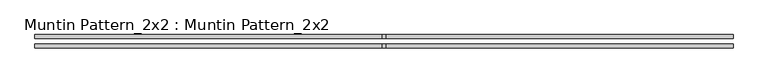
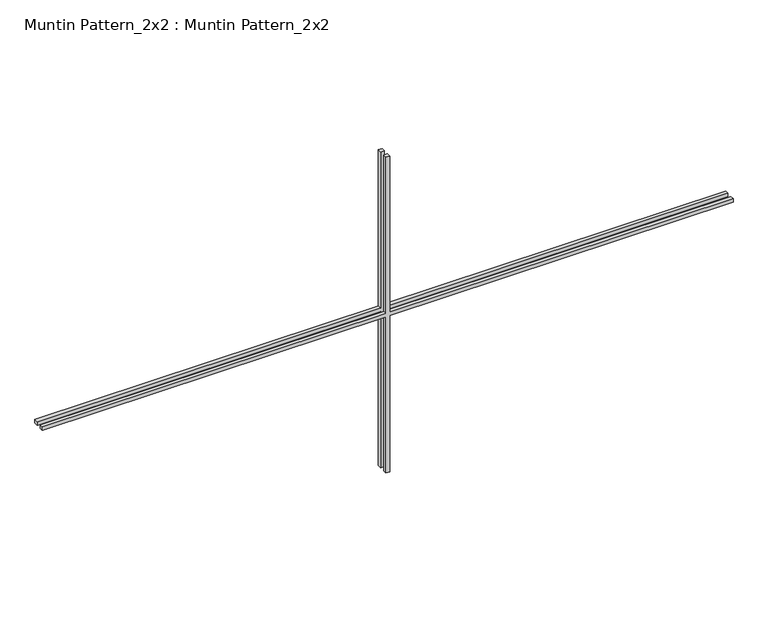
"""IFC4 building model written with IfcOpenShell, lengths in millimetres: proxy geometry, Muntin Pattern_2x2 : Muntin Pattern_2x2."""

from ifc_helpers import new_model, si_unit, frame, origin, place, context, project, spatial, polyline, outline, extrude, source, transform, mapped, element, save


def muntin_pattern_2x2_muntin_pattern_2x2_6be186e8(model_context):
    return source(origin(), model_context, "Body", "SweptSolid", [
        extrude(outline(polyline([(577.85, -6.35), (577.85, -1181.1), (565.15, -1181.1), (565.15, -6.35), (0.0, -6.35), (0.0, 6.35), (565.15, 6.35), (565.15, 1181.1), (577.85, 1181.1), (577.85, 6.35), (1143.0, 6.35), (1143.0, -6.35), (577.85, -6.35)])), frame((0.0, -22.225, 0.0), z_axis=(0.0, 1.0, 0.0), x_axis=(0.0, 0.0, 1.0)), (0.0, 0.0, 1.0), 12.7),
        extrude(outline(polyline([(577.85, -6.35), (577.85, -1181.1), (565.15, -1181.1), (565.15, -6.35), (0.0, -6.35), (0.0, 6.35), (565.15, 6.35), (565.15, 1181.1), (577.85, 1181.1), (577.85, 6.35), (1143.0, 6.35), (1143.0, -6.35), (577.85, -6.35)])), frame((0.0, 9.525, 0.0), z_axis=(0.0, 1.0, 0.0), x_axis=(0.0, 0.0, 1.0)), (0.0, 0.0, 1.0), 12.7),
    ])


if __name__ == "__main__":
    model = new_model("IFC4")
    model_context = context("Model", 3, world=origin())
    ifc_project = project(units=[si_unit("LENGTHUNIT", "METRE", prefix="MILLI")], contexts=[model_context])
    site = spatial("IfcSite", under=ifc_project)
    building = spatial("IfcBuilding", under=site)
    placement = place(None, origin())
    muntin_pattern_2x2_muntin_pattern_2x2_shape = muntin_pattern_2x2_muntin_pattern_2x2_6be186e8(model_context)
    element("IfcBuildingElementProxy", 1, Name="Muntin Pattern_2x2 : Muntin Pattern_2x2", ObjectType="Muntin Pattern_2x2 : Muntin Pattern_2x2", at=placement, inside=building, context=model_context, shape_type="MappedRepresentation", body=[
        mapped(muntin_pattern_2x2_muntin_pattern_2x2_shape, transform((0.0, 0.0, 0.0), x_axis=(1.0, 0.0, 0.0), y_axis=(0.0, 1.0, 0.0), z_axis=(0.0, 0.0, 1.0))),
    ])
    save(model, "model.ifc")

# Revit data of these elements
# Type "Muntin Pattern_2x2 : Muntin Pattern_2x2"
#   Width [instance default] = 4' - 0"
#   Thickness = 0' - 0 1/2"
#   Height [instance default] = 4' - 0"
#   Distance = 0' - 0 3/4"
#   Interior Material [instance default] = none
#   Exterior Material [instance default] = none
#   Default Elevation = 0
# Element 1 (IfcBuildingElementProxy, "Muntin Pattern_2x2 : Muntin Pattern_2x2")
#   Width = 7' - 9"
#   Height = 3' - 9"
#   Interior Material = Wood - Stained
#   Exterior Material = Clad - White
#   Materials on its faces: "Clad - White", "Wood - Stained"
# Materials
#   "Clad - White": class "Wood", colour RGB 242 242 238, transparency 0, Cost = 0
#   "Wood - Stained": class "Wood", colour RGB 224 178 126, transparency 0, Cost = 0
